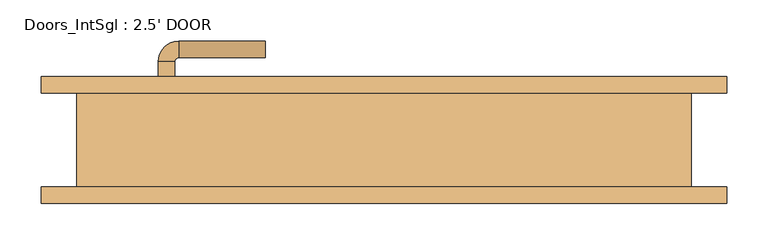
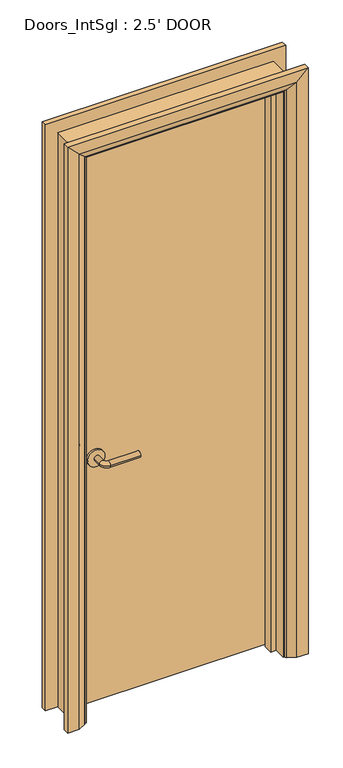
"""IFC4 building model written with IfcOpenShell, lengths in millimetres: door geometry, Doors_IntSgl : 2.5' DOOR."""

from ifc_helpers import new_model, si_unit, point, frame, frame_2d, origin, place, context, project, spatial, polyline, circle_curve, ellipse_curve, trimmed, segment, composite_curve, outline, extrude, faceted_brep, source, transform, mapped, element, save
from ifc_brep_helpers import plane_surface, cylinder_surface, revolved_surface, advanced_brep


def doors_intsgl_2_5_door_21b53886(model_context):
    return source(origin(), model_context, "Body", "SolidModel", [
        advanced_brep(
        [(-274.0, 11.15, 900.0), (-254.0, 11.15, 900.0), (-254.0, -18.85, 900.0), (-274.0, -18.85, 900.0), (-249.0, -23.85, 900.0), (-249.0, -43.85, 900.0), (-144.0, -43.85, 900.0), (-144.0, -23.85, 900.0)],
        [
            (0, 1, circle_curve(frame((-264.0, 11.15, 900.0), z_axis=(0.0, 1.0, 0.0), x_axis=(1.0, 0.0, 0.0)), 10.0)),
            (1, 0, circle_curve(frame((-264.0, 11.15, 900.0), z_axis=(0.0, 1.0, 0.0), x_axis=(1.0, 0.0, 0.0)), 10.0)),
            (1, 2),
            (2, 3, circle_curve(frame((-264.0, -18.85, 900.0), z_axis=(0.0, 1.0, 0.0), x_axis=(1.0, 0.0, 0.0)), 10.0)),
            (3, 0),
            (3, 2, circle_curve(frame((-264.0, -18.85, 900.0), z_axis=(0.0, 1.0, 0.0), x_axis=(1.0, 0.0, 0.0)), 10.0)),
            (4, 5, circle_curve(frame((-249.0, -33.85, 900.0), z_axis=(-1.0, 0.0, 0.0), x_axis=(0.0, 1.0, 0.0)), 10.0)),
            (5, 3, circle_curve(frame((-249.0, -18.85, 900.0), z_axis=(0.0, 0.0, -1.0), x_axis=(-1.0, 0.0, 0.0)), 25.0)),
            (2, 4, circle_curve(frame((-249.0, -18.85, 900.0), z_axis=(0.0, 0.0, 1.0), x_axis=(-1.0, 0.0, 0.0)), 5.0)),
            (5, 4, circle_curve(frame((-249.0, -33.85, 900.0), z_axis=(-1.0, 0.0, 0.0), x_axis=(0.0, 1.0, 0.0)), 10.0)),
            (6, 7, circle_curve(frame((-144.0, -33.85, 900.0), z_axis=(1.0, 0.0, 0.0), x_axis=(0.0, 1.0, 0.0)), 10.0)),
            (7, 6, circle_curve(frame((-144.0, -33.85, 900.0), z_axis=(1.0, 0.0, 0.0), x_axis=(0.0, 1.0, 0.0)), 10.0)),
            (4, 7),
            (6, 5),
        ],
        [
            plane_surface(frame((-264.0, 11.15, 900.0), z_axis=(0.0, 1.0, 0.0), x_axis=(0.0, 0.0, 1.0))),
            cylinder_surface(frame((-264.0, 11.15, 900.0), z_axis=(0.0, 1.0, 0.0), x_axis=(1.0, 0.0, 0.0)), 10.0),
            revolved_surface(trimmed(ellipse_curve(frame((-264.0, -18.85, 900.0), z_axis=(0.0, -1.0, 0.0), x_axis=(1.0, 0.0, 0.0)), 10.0, 10.0), [point((-274.0, -18.85, 900.0))], [point((-254.0, -18.85, 900.0))], True, "CARTESIAN"), (-249.0, -18.85, 900.0), (0.0, 0.0, -1.0)),
            revolved_surface(trimmed(ellipse_curve(frame((-264.0, -18.85, 900.0), z_axis=(0.0, -1.0, 0.0), x_axis=(1.0, 0.0, 0.0)), 10.0, 10.0), [point((-254.0, -18.85, 900.0))], [point((-274.0, -18.85, 900.0))], True, "CARTESIAN"), (-249.0, -18.85, 900.0), (0.0, 0.0, -1.0)),
            plane_surface(frame((-144.0, -33.85, 900.0), z_axis=(1.0, 0.0, 0.0), x_axis=(0.0, 0.0, 1.0))),
            cylinder_surface(frame((-249.0, -33.85, 900.0), z_axis=(-1.0, 0.0, 0.0), x_axis=(0.0, 1.0, 0.0)), 10.0),
        ],
        [
            (0, [[1, 2]]),
            (1, [[3, 4, 5, -2]]),
            (1, [[-5, 6, -3, -1]]),
            (2, [[7, 8, -4, 9]]),
            (3, [[10, -9, -6, -8]]),
            (4, [[11, 12]]),
            (5, [[13, -11, 14, -7]]),
            (5, [[-14, -12, -13, -10]]),
        ],
    ),
        extrude(outline(composite_curve([segment(trimmed(circle_curve(frame_2d((900.0, -266.5)), 30.0), [point((900.0, -296.5))], [point((900.0, -236.5))], False, "CARTESIAN"), True, "CONTINUOUS"), segment(trimmed(circle_curve(frame_2d((900.0, -266.5)), 30.0), [point((900.0, -236.5))], [point((900.0, -296.5))], False, "CARTESIAN"), True, "CONTINUOUS")], self_intersect=False)), frame((0.0, 11.15, 0.0), z_axis=(0.0, 1.0, 0.0), x_axis=(0.0, 0.0, 1.0)), (0.0, 0.0, 1.0), 8.0),
        advanced_brep(
        [(-274.0, 65.15, 900.0), (-254.0, 65.15, 900.0), (-274.0, 95.15, 900.0), (-254.0, 95.15, 900.0), (-249.0, 100.15, 900.0), (-249.0, 120.15, 900.0), (-144.0, 120.15, 900.0), (-144.0, 100.15, 900.0)],
        [
            (0, 1, circle_curve(frame((-264.0, 65.15, 900.0), z_axis=(0.0, -1.0, 0.0), x_axis=(1.0, 0.0, 0.0)), 10.0)),
            (1, 0, circle_curve(frame((-264.0, 65.15, 900.0), z_axis=(0.0, -1.0, 0.0), x_axis=(1.0, 0.0, 0.0)), 10.0)),
            (0, 2),
            (2, 3, circle_curve(frame((-264.0, 95.15, 900.0), z_axis=(0.0, -1.0, 0.0), x_axis=(1.0, 0.0, 0.0)), 10.0)),
            (3, 1),
            (3, 2, circle_curve(frame((-264.0, 95.15, 900.0), z_axis=(0.0, -1.0, 0.0), x_axis=(1.0, 0.0, 0.0)), 10.0)),
            (4, 3, circle_curve(frame((-249.0, 95.15, 900.0), z_axis=(0.0, 0.0, 1.0), x_axis=(-1.0, 0.0, 0.0)), 5.0)),
            (2, 5, circle_curve(frame((-249.0, 95.15, 900.0), z_axis=(0.0, 0.0, -1.0), x_axis=(-1.0, 0.0, 0.0)), 25.0)),
            (5, 4, circle_curve(frame((-249.0, 110.15, 900.0), z_axis=(-1.0, 0.0, 0.0), x_axis=(0.0, -1.0, 0.0)), 10.0)),
            (4, 5, circle_curve(frame((-249.0, 110.15, 900.0), z_axis=(-1.0, 0.0, 0.0), x_axis=(0.0, -1.0, 0.0)), 10.0)),
            (6, 7, circle_curve(frame((-144.0, 110.15, 900.0), z_axis=(1.0, 0.0, 0.0), x_axis=(0.0, -1.0, 0.0)), 10.0)),
            (7, 6, circle_curve(frame((-144.0, 110.15, 900.0), z_axis=(1.0, 0.0, 0.0), x_axis=(0.0, -1.0, 0.0)), 10.0)),
            (5, 6),
            (7, 4),
        ],
        [
            plane_surface(frame((-264.0, 65.15, 900.0), z_axis=(0.0, -1.0, 0.0), x_axis=(0.0, 0.0, 1.0))),
            cylinder_surface(frame((-264.0, 65.15, 900.0), z_axis=(0.0, -1.0, 0.0), x_axis=(1.0, 0.0, 0.0)), 10.0),
            revolved_surface(trimmed(ellipse_curve(frame((-264.0, 95.15, 900.0), z_axis=(0.0, -1.0, 0.0), x_axis=(1.0, 0.0, 0.0)), 10.0, 10.0), [point((-274.0, 95.15, 900.0))], [point((-254.0, 95.15, 900.0))], True, "CARTESIAN"), (-249.0, 95.15, 900.0), (0.0, 0.0, -1.0)),
            revolved_surface(trimmed(ellipse_curve(frame((-264.0, 95.15, 900.0), z_axis=(0.0, -1.0, 0.0), x_axis=(1.0, 0.0, 0.0)), 10.0, 10.0), [point((-254.0, 95.15, 900.0))], [point((-274.0, 95.15, 900.0))], True, "CARTESIAN"), (-249.0, 95.15, 900.0), (0.0, 0.0, -1.0)),
            plane_surface(frame((-144.0, 110.15, 900.0), z_axis=(1.0, 0.0, 0.0), x_axis=(0.0, 0.0, 1.0))),
            cylinder_surface(frame((-249.0, 110.15, 900.0), z_axis=(-1.0, 0.0, 0.0), x_axis=(0.0, -1.0, 0.0)), 10.0),
        ],
        [
            (0, [[1, 2]]),
            (1, [[-1, 3, 4, 5]]),
            (1, [[-2, -5, 6, -3]]),
            (2, [[7, -4, 8, 9]]),
            (3, [[-8, -6, -7, 10]]),
            (4, [[11, 12]]),
            (5, [[-9, 13, -12, 14]]),
            (5, [[-10, -14, -11, -13]]),
        ],
    ),
        extrude(outline(composite_curve([segment(trimmed(circle_curve(frame_2d((900.0, -266.5)), 30.0), [point((900.0, -296.5))], [point((900.0, -236.5))], False, "CARTESIAN"), True, "CONTINUOUS"), segment(trimmed(circle_curve(frame_2d((900.0, -266.5)), 30.0), [point((900.0, -236.5))], [point((900.0, -296.5))], False, "CARTESIAN"), True, "CONTINUOUS")], self_intersect=False)), frame((0.0, 57.15, 0.0), z_axis=(0.0, 1.0, 0.0), x_axis=(0.0, 0.0, 1.0)), (0.0, 0.0, 1.0), 8.0),
        extrude(outline(polyline([(339.0, 19.15), (-339.0, 19.15), (-339.0, 57.15), (339.0, 57.15), (339.0, 19.15)])), frame((0.0, 0.0, 8.0), z_axis=(0.0, 0.0, 1.0), x_axis=(1.0, 0.0, 0.0)), (0.0, 0.0, 1.0), 2060.0),
        advanced_brep(
        [(416.0, 77.15, 0.0), (416.0, 57.15, 0.0), (346.0, 57.15, 0.0), (350.0, 63.15, 0.0), (376.0, 77.15, 0.0), (416.0, 77.15, 2145.0), (416.0, 57.15, 2145.0), (-416.0, 57.15, 2145.0), (-416.0, 57.15, 0.0), (-346.0, 57.15, 0.0), (-346.0, 57.15, 2075.0), (346.0, 57.15, 2075.0), (350.0, 63.15, 2079.0), (376.0, 77.15, 2105.0), (-376.0, 77.15, 2105.0), (-376.0, 77.15, 0.0), (-416.0, 77.15, 0.0), (-416.0, 77.15, 2145.0), (-350.0, 63.15, 0.0), (-350.0, 63.15, 2079.0)],
        [
            (0, 1),
            (1, 2),
            (2, 3, circle_curve(frame((354.0, 56.15, 0.0), z_axis=(0.0, 0.0, -1.0), x_axis=(1.0, 0.0, 0.0)), 8.0622577)),
            (3, 4),
            (4, 0),
            (0, 5),
            (5, 6),
            (6, 1),
            (6, 7),
            (7, 8),
            (8, 9),
            (9, 10),
            (10, 11),
            (11, 2),
            (11, 12, ellipse_curve(frame((354.0, 56.15, 2083.0), z_axis=(0.7071067811865475, 0.0, -0.7071067811865475), x_axis=(-0.7071067811865474, 0.0, -0.7071067811865476)), 11.4017543, 8.0622577)),
            (12, 3),
            (12, 13),
            (13, 4),
            (13, 14),
            (14, 15),
            (15, 16),
            (16, 17),
            (17, 5),
            (7, 17),
            (16, 8),
            (15, 18),
            (18, 9, circle_curve(frame((-354.0, 56.15, 0.0), z_axis=(0.0, 0.0, -1.0), x_axis=(-1.0, 0.0, 0.0)), 8.0622577)),
            (19, 10, ellipse_curve(frame((-354.0, 56.15, 2083.0), z_axis=(-0.7071067811865475, 0.0, -0.7071067811865475), x_axis=(-0.7071067811865474, 0.0, 0.7071067811865476)), 11.4017543, 8.0622577)),
            (18, 19),
            (14, 19),
            (19, 12),
        ],
        [
            plane_surface(frame((346.0, 57.15, 0.0), z_axis=(0.0, 0.0, -1.0), x_axis=(0.0, -1.0, 0.0))),
            plane_surface(frame((416.0, 77.15, 0.0), z_axis=(1.0, 0.0, 0.0), x_axis=(0.0, 0.0, 1.0))),
            plane_surface(frame((416.0, 57.15, 0.0), z_axis=(0.0, -1.0, 0.0), x_axis=(0.0, 0.0, 1.0))),
            cylinder_surface(frame((354.0, 56.15, 0.0), z_axis=(0.0, 0.0, -1.0), x_axis=(1.0, 0.0, 0.0)), 8.0622577),
            plane_surface(frame((350.0, 63.15, 0.0), z_axis=(-0.4740998230350126, 0.880471099922178, 0.0), x_axis=(0.0, 0.0, 1.0))),
            plane_surface(frame((376.0, 77.15, 0.0), z_axis=(0.0, 1.0, 0.0), x_axis=(0.0, 0.0, 1.0))),
            plane_surface(frame((-416.0, 77.15, 2145.0), z_axis=(-1.0, 0.0, 0.0), x_axis=(0.0, 0.0, -1.0))),
            plane_surface(frame((-346.0, 57.15, 0.0), z_axis=(0.0, 0.0, -1.0), x_axis=(0.0, -1.0, 0.0))),
            cylinder_surface(frame((-354.0, 56.15, 2075.0), z_axis=(0.0, 0.0, 1.0), x_axis=(-1.0, 0.0, 0.0)), 8.0622577),
            plane_surface(frame((-350.0, 63.15, 2079.0), z_axis=(0.47409982303501824, 0.8804710999221749, 0.0), x_axis=(0.0, 0.0, -1.0))),
            plane_surface(frame((416.0, 77.15, 2145.0), z_axis=(0.0, 0.0, 1.0), x_axis=(-1.0, 0.0, 0.0))),
            cylinder_surface(frame((346.0, 56.15, 2083.0), z_axis=(1.0, 0.0, 0.0), x_axis=(0.0, 0.0, 1.0)), 8.0622577),
            plane_surface(frame((350.0, 63.15, 2079.0), z_axis=(0.0, 0.8804710999221764, -0.4740998230350154), x_axis=(-1.0, 0.0, 0.0))),
        ],
        [
            (0, [[1, 2, 3, 4, 5]]),
            (1, [[-1, 6, 7, 8]]),
            (2, [[-2, -8, 9, 10, 11, 12, 13, 14]]),
            (3, [[-3, -14, 15, 16]]),
            (4, [[-4, -16, 17, 18]]),
            (5, [[-5, -18, 19, 20, 21, 22, 23, -6]]),
            (6, [[24, -22, 25, -10]]),
            (7, [[-21, 26, 27, -11, -25]]),
            (8, [[28, -12, -27, 29]]),
            (9, [[30, -29, -26, -20]]),
            (10, [[-7, -23, -24, -9]]),
            (11, [[-15, -13, -28, 31]]),
            (12, [[-17, -31, -30, -19]]),
        ],
    ),
        extrude(outline(polyline([(0.0, -341.0), (0.0, -322.0), (2051.0, -322.0), (2051.0, 322.0), (0.0, 322.0), (0.0, 341.0), (2070.0, 341.0), (2070.0, -341.0), (0.0, -341.0)])), frame((0.0, -14.85, 0.0), z_axis=(0.0, 1.0, 0.0), x_axis=(0.0, 0.0, 1.0)), (0.0, 0.0, 1.0), 32.0),
        advanced_brep(
        [(-416.0, -77.15, 0.0), (-416.0, -57.15, 0.0), (-346.0, -57.15, 0.0), (-350.0, -63.15, 0.0), (-376.0, -77.15, 0.0), (-416.0, -77.15, 2145.0), (-416.0, -57.15, 2145.0), (-346.0, -57.15, 2075.0), (-350.0, -63.15, 2079.0), (-376.0, -77.15, 2105.0), (416.0, -77.15, 0.0), (376.0, -77.15, 0.0), (350.0, -63.15, 0.0), (346.0, -57.15, 0.0), (416.0, -57.15, 0.0), (416.0, -77.15, 2145.0), (376.0, -77.15, 2105.0), (350.0, -63.15, 2079.0), (346.0, -57.15, 2075.0), (416.0, -57.15, 2145.0)],
        [
            (0, 1),
            (1, 2),
            (2, 3, circle_curve(frame((-354.0, -56.15, 0.0), z_axis=(0.0, 0.0, -1.0), x_axis=(-1.0, 0.0, 0.0)), 8.0622577)),
            (3, 4),
            (4, 0),
            (0, 5),
            (5, 6),
            (6, 1),
            (6, 7),
            (7, 2),
            (7, 8, ellipse_curve(frame((-354.0, -56.15, 2083.0), z_axis=(-0.7071067811865475, 0.0, -0.7071067811865475), x_axis=(0.7071067811865474, 0.0, -0.7071067811865476)), 11.4017543, 8.0622577)),
            (8, 3),
            (8, 9),
            (9, 4),
            (9, 5),
            (10, 11),
            (11, 12),
            (12, 13, circle_curve(frame((354.0, -56.15, 0.0), z_axis=(0.0, 0.0, -1.0), x_axis=(1.0, 0.0, 0.0)), 8.0622577)),
            (13, 14),
            (14, 10),
            (15, 16),
            (16, 11),
            (10, 15),
            (16, 17),
            (17, 12),
            (17, 18, ellipse_curve(frame((354.0, -56.15, 2083.0), z_axis=(0.7071067811865475, 0.0, -0.7071067811865475), x_axis=(0.7071067811865474, 0.0, 0.7071067811865476)), 11.4017543, 8.0622577)),
            (18, 13),
            (18, 19),
            (19, 14),
            (19, 15),
            (5, 15),
            (19, 6),
            (18, 7),
            (17, 8),
            (16, 9),
        ],
        [
            plane_surface(frame((-346.0, -129.9510989, 0.0), z_axis=(0.0, 0.0, -1.0), x_axis=(1.0, 0.0, 0.0))),
            plane_surface(frame((-416.0, -77.15, 0.0), z_axis=(-1.0, 0.0, 0.0), x_axis=(0.0, 0.0, 1.0))),
            plane_surface(frame((-416.0, -57.15, 0.0), z_axis=(0.0, 1.0, 0.0), x_axis=(0.0, 0.0, 1.0))),
            cylinder_surface(frame((-354.0, -56.15, 0.0), z_axis=(0.0, 0.0, -1.0), x_axis=(-1.0, 0.0, 0.0)), 8.0622577),
            plane_surface(frame((-350.0, -63.15, 0.0), z_axis=(0.4740998230350183, -0.8804710999221749, 0.0), x_axis=(0.0, 0.0, 1.0))),
            plane_surface(frame((-376.0, -77.15, 0.0), z_axis=(0.0, -1.0, 0.0), x_axis=(0.0, 0.0, 1.0))),
            plane_surface(frame((346.0, -129.9510989, 0.0), z_axis=(0.0, 0.0, -1.0), x_axis=(-1.0, 0.0, 0.0))),
            plane_surface(frame((376.0, -77.15, 2105.0), z_axis=(0.0, -1.0, 0.0), x_axis=(0.0, 0.0, -1.0))),
            plane_surface(frame((350.0, -63.15, 2079.0), z_axis=(-0.4740998230350183, -0.8804710999221749, 0.0), x_axis=(0.0, 0.0, -1.0))),
            cylinder_surface(frame((354.0, -56.15, 2075.0), z_axis=(0.0, 0.0, 1.0), x_axis=(1.0, 0.0, 0.0)), 8.0622577),
            plane_surface(frame((416.0, -57.15, 2145.0), z_axis=(0.0, 1.0, 0.0), x_axis=(0.0, 0.0, -1.0))),
            plane_surface(frame((416.0, -77.15, 2145.0), z_axis=(1.0, 0.0, 0.0), x_axis=(0.0, 0.0, -1.0))),
            plane_surface(frame((-416.0, -77.15, 2145.0), z_axis=(0.0, 0.0, 1.0), x_axis=(1.0, 0.0, 0.0))),
            plane_surface(frame((-416.0, -57.15, 2145.0), z_axis=(0.0, 1.0, 0.0), x_axis=(1.0, 0.0, 0.0))),
            cylinder_surface(frame((-346.0, -56.15, 2083.0), z_axis=(-1.0, 0.0, 0.0), x_axis=(0.0, 0.0, 1.0)), 8.0622577),
            plane_surface(frame((-350.0, -63.15, 2079.0), z_axis=(0.0, -0.8804710999221749, -0.4740998230350183), x_axis=(1.0, 0.0, 0.0))),
            plane_surface(frame((-376.0, -77.15, 2105.0), z_axis=(0.0, -1.0, 0.0), x_axis=(1.0, 0.0, 0.0))),
        ],
        [
            (0, [[1, 2, 3, 4, 5]]),
            (1, [[-1, 6, 7, 8]]),
            (2, [[-2, -8, 9, 10]]),
            (3, [[-3, -10, 11, 12]]),
            (4, [[-4, -12, 13, 14]]),
            (5, [[-5, -14, 15, -6]]),
            (6, [[16, 17, 18, 19, 20]]),
            (7, [[21, 22, -16, 23]]),
            (8, [[24, 25, -17, -22]]),
            (9, [[26, 27, -18, -25]]),
            (10, [[28, 29, -19, -27]]),
            (11, [[30, -23, -20, -29]]),
            (12, [[-7, 31, -30, 32]]),
            (13, [[-9, -32, -28, 33]]),
            (14, [[-11, -33, -26, 34]]),
            (15, [[-13, -34, -24, 35]]),
            (16, [[-15, -35, -21, -31]]),
        ],
    ),
        faceted_brep([(-341.0, 57.15, 0.0), (-341.0, -57.15, 0.0), (-373.0, -57.15, 0.0), (-373.0, 57.15, 0.0), (-341.0, 57.15, 2070.0), (-341.0, -57.15, 2070.0), (-373.0, -57.15, 2102.0), (-373.0, 57.15, 2102.0), (341.0, 57.15, 0.0), (373.0, 57.15, 0.0), (373.0, -57.15, 0.0), (341.0, -57.15, 0.0), (341.0, 57.15, 2070.0), (373.0, 57.15, 2102.0), (373.0, -57.15, 2102.0), (341.0, -57.15, 2070.0)], [[[0, 1, 2, 3]], [[1, 0, 4, 5]], [[2, 1, 5, 6]], [[3, 2, 6, 7]], [[0, 3, 7, 4]], [[8, 9, 10, 11]], [[12, 13, 9, 8]], [[13, 14, 10, 9]], [[14, 15, 11, 10]], [[15, 12, 8, 11]], [[5, 4, 12, 15]], [[6, 5, 15, 14]], [[7, 6, 14, 13]], [[4, 7, 13, 12]]]),
    ])


if __name__ == "__main__":
    model = new_model("IFC4")
    model_context = context("Model", 3, world=origin())
    ifc_project = project(units=[si_unit("LENGTHUNIT", "METRE", prefix="MILLI")], contexts=[model_context])
    site = spatial("IfcSite", under=ifc_project)
    building = spatial("IfcBuilding", under=site)
    placement = place(None, origin())
    doors_intsgl_2_5_door_shape = doors_intsgl_2_5_door_21b53886(model_context)
    element("IfcDoor", 1, ObjectType="Doors_IntSgl : 2.5' DOOR", at=placement, inside=building, context=model_context, shape_type="MappedRepresentation", body=[
        mapped(doors_intsgl_2_5_door_shape, transform((0.0, 0.0, 0.0), x_axis=(1.0, 0.0, 0.0), y_axis=(0.0, 1.0, 0.0), z_axis=(0.0, 0.0, 1.0))),
    ])
    save(model, "model.ifc")

# Revit data of these elements
# Type "Doors_IntSgl : 2.5' DOOR"
#   Type Mark = "47"
#   Type Comments = "Internal Single"
#   Operation = "SingleSwingRight"
#   Manufacturer = "Revit"
#   Keynote = "L20"
#   Description = "Internal Single Door"
#   Analytic Construction = "Metal"
#   UnderCut = 0.026247 ft
#   Tolerance = 0.006562 ft
#   Thickness = 0.124672 ft
#   Thermal Resistance (R) = 0.270117 (m²·K)/W
#   Structural Tolerance = 0.026247 ft
#   StopDepth = 0.104987 ft
#   Stop Thickness = 0.062336 ft
#   Rough Width = 2.5 ft
#   Rough Height = 6.922572 ft
#   Height to Top Lock Rail = 3.28084 ft
#   Heat Transfer Coefficient (U) = 3.7021 W/(m²·K)
#   Handle Z Distance = 2.952756 ft
#   Handle X Distance = 0.246063 ft
#   Frame Thickness = 0.104987 ft
#   Door Panel Width = 2.224409 ft
#   Door Panel Thickness = 0.124672 ft
#   Door Panel Offset = 0.0 ft
#   Height = 6.922572 ft
#   Width = 2.5 ft
#   Door Panel Height = 6.75853 ft
#   Architrave Setback = 0.016404 ft
#   Vis - Ironmongery = yes
#   Material Ironmongery = Door - Handle
#   Material Frame = Door - Frame/Mullion (1)
#   Material Door = Door - Panel
#   Material Architrave = Door - Architrave
#   Visual Light Transmittance = 0
#   Solar Heat Gain Coefficient = 0
#   Function = (empty or 0)
#   Wall Closure = (empty or 0)
# Element 1 (IfcDoor, "Doors_IntSgl : 2.5' DOOR")
#   Materials on its faces: "Door - Architrave", "Door - Handle", "Door - Frame/Mullion (1)", "Door - Panel"
# Materials
#   "Door - Handle": colour RGB 0 0 0, transparency 0, Keynote = "P21", Cost = 0
#   "Door - Frame/Mullion (1)": class "Wood", colour RGB 212 179 113, transparency 0, Keynote = "L20", Cost = 0
#   "Door - Panel": class "Wood", colour RGB 210 159 95, transparency 0, Keynote = "L20", Cost = 0
#   "Door - Architrave": class "Wood", colour RGB 154 90 5, transparency 0, Keynote = "P20", Cost = 0
